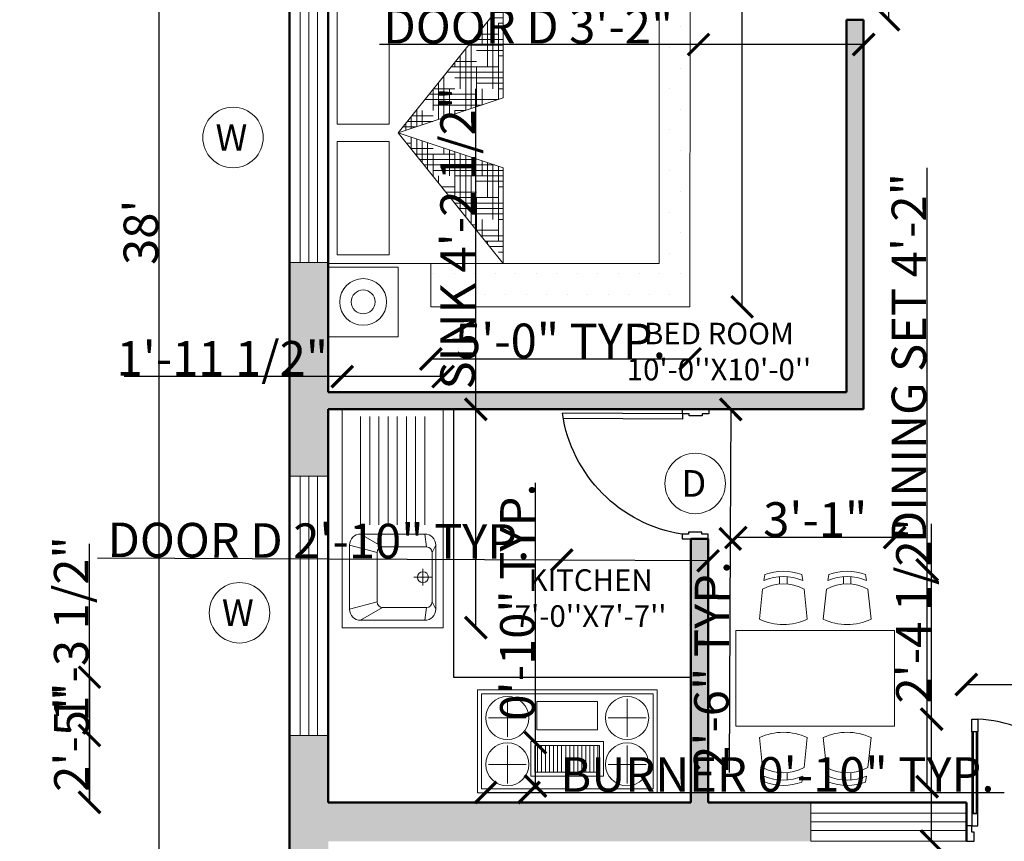
# Model space of a CAD drawing. Units: inches. Extents: x 1938 to 2373, y 1634 to 2225.
# Tile 2 of 5: x 1938 to 2166, y 1755 to 1945. Entities that reach past the tile are written whole.
import ezdxf

# ---------------------------------------------------------------- set-up
doc = ezdxf.new("R2010")
doc.units = ezdxf.units.IN
for name, color, linetype, lineweight in [('A-ANNO-DIMS', 2, 'Continuous', 18), ('A-ANNO-SYMB', 7, 'Continuous', 18), ('A-AREA-IDEN', 7, 'Continuous', 18), ('A-EQPM', 8, 'Continuous', 18), ('A-EQPM-PATT', 8, 'Continuous', 13), ('A-FLOR-FIXT', 9, 'Continuous', 18), ('A-FURN', 8, 'Continuous', 18), ('A-FURN-PATT', 7, 'Continuous', 13), ('A-WALL-PATT', 82, 'Continuous', 13), ('DOOR', 30, 'Continuous', 25), ('KITCHEN', 40, 'Continuous', 25), ('MAIN DOOR', 150, 'Continuous', 25), ('WALL', 7, 'Continuous', 50), ('WINDOW', 150, 'Continuous', 18)]:
    doc.layers.add(name, color=color, linetype=linetype, lineweight=lineweight)
doc.layers.add('A-Glaz', color=92, linetype='Continuous')
doc.styles.get("Standard").update_dxf_attribs({"font": 'arial.ttf'})
doc.dimstyles.get("Standard").update_dxf_attribs({"dimtxt": 8, "dimasz": 5, "dimexe": 0.18, "dimexo": 0.0625, "dimgap": 0.09, "dimtad": 1, "dimdec": 1, "dimzin": 0, "dimdsep": 46, "dimlunit": 4, "dimtxsty": 'Standard', "dimblk": 'ARCHTICK', "dimcen": 0.09, "dimse1": 1, "dimse2": 1, "dimadec": 0, "dimazin": 0, "dimtfac": 1, "dimtdec": 1, "dimtofl": 0, "dimtmove": 0, "dimatfit": 3, "dimfxl": 1, "dimtolj": 1, "dimtzin": 0, "dimarcsym": 0})

# ---------------------------------------------------------------- blocks, each defined once
blk = doc.blocks.new('A$C13CE0A17')
at = {"layer": 'A-Glaz'}
for p, q in [((0.01, 0.61), (0.01, 0.08)), ((0.03, 0.08), (0.03, 0.61))]:
    blk.add_line(p, q, dxfattribs=at)
blk.add_lwpolyline([(1.4, 0.08), (1.4, 0.61), (1.42, 0.61), (1.42, 0.08)], close=True, dxfattribs=at)
at = {"layer": 'MAIN DOOR'}
for p, q in [((0, 0.61), (0, 0.69)), ((0, 0.69), (0.04, 0.69)), ((0.04, 0.69), (0.04, 0.61)), ((0, 0.61), (0, 0.08)), ((0.04, 0.61), (0, 0.61)), ((0.04, 0.61), (0, 0.61)), ((0.03, 0.61), (0.01, 0.61)), ((0.04, 0.08), (0.04, 0.61)), ((0, 0.08), (0, 0)), ((0.04, 0.08), (0, 0.08)), ((0, 0.08), (0.04, 0.08)), ((0.01, 0.08), (0.03, 0.08)), ((0.04, 0), (0.04, 0.08)), ((-0.035, 0), (-0.035, -0.1)), ((0, 0), (-0.035, 0)), ((0, 0), (0.04, 0)), ((0, -0.04), (0, 0)), ((0.015, -0.04), (0, -0.04)), ((0.015, -0.05), (0.015, -0.04)), ((0.015, -0.1), (0.015, -0.05)), ((-0.035, -0.1), (0.015, -0.1))]:
    blk.add_line(p, q, dxfattribs=at)
for points in [[(1.39, 0.69), (1.39, 0.61), (1.43, 0.61), (1.43, 0.69)], [(1.39, 0.08), (1.39, 0.61), (1.43, 0.61), (1.43, 0.08)], [(1.39, 0), (1.39, 0.08), (1.43, 0.08), (1.43, 0)], [(1.43, 0), (1.465, 0), (1.465, -0.1), (1.415, -0.1), (1.415, -0.05), (1.415, -0.04), (1.43, -0.04)]]:
    blk.add_lwpolyline(points, close=True, dxfattribs=at)
blk.add_arc((1.3872, 0.017), 0.673, 89.76573, 181.44381, dxfattribs=at)
blk.add_ellipse((0.0389, 0.0511), major_axis=(0.6669, -0.1217), ratio=0.940794, start_param=0.11153, end_param=1.73917, dxfattribs=at)
blk = doc.blocks.new('table-23')
at = {"color": 0, "linetype": 'ByBlock'}
for p, q in [((-0.9, -1.4923), (-0.9, 0)), ((-0.9, 0), (0, 0)), ((0, -1.4923), (0, 0)), ((-1.3677, -0.2639), (-1.4237, -0.2726)), ((-1.0062, -0.2211), (-1.2862, -0.2511)), ((0.1062, -0.2211), (0.3862, -0.2511)), ((0.4677, -0.2639), (0.5237, -0.2726)), ((-1.4049, -0.4111), (-1.3347, -0.4111)), ((0.5049, -0.4111), (0.4347, -0.4111)), ((-1.4049, -0.4811), (-1.3347, -0.4811)), ((0.5049, -0.4811), (0.4347, -0.4811)), ((-1.3677, -0.6284), (-1.4237, -0.6197)), ((-1.0062, -0.6711), (-1.2862, -0.6411)), ((0.1062, -0.6711), (0.3862, -0.6411)), ((0.4677, -0.6284), (0.5237, -0.6197)), ((-1.0062, -0.8211), (-1.2862, -0.8511)), ((0.1062, -0.8211), (0.3862, -0.8511)), ((-1.3677, -0.8639), (-1.4237, -0.8726)), ((0.4677, -0.8639), (0.5237, -0.8726)), ((-1.4049, -1.0111), (-1.3347, -1.0111)), ((0.5049, -1.0111), (0.4347, -1.0111)), ((-1.4049, -1.0811), (-1.3347, -1.0811)), ((0.5049, -1.0811), (0.4347, -1.0811)), ((-1.3677, -1.2284), (-1.4237, -1.2197)), ((-1.0062, -1.2711), (-1.2862, -1.2411)), ((0.1062, -1.2711), (0.3862, -1.2411)), ((0.4677, -1.2284), (0.5237, -1.2197)), ((-0.9, -1.4923), (0, -1.4923))]:
    blk.add_line(p, q, dxfattribs=at)
for centre, radius, start, end in [((-0.9765, -0.4461), 0.4797, 158.78869, 201.21131), ((-0.9558, -0.4461), 0.4505, 156.13443, 203.86557), ((-0.931, -0.4461), 0.4053, 151.23721, 208.76279), ((-1.4875, -0.4461), 0.5312, 334.94238, 25.05762), ((0.5875, -0.4461), 0.5312, 154.94238, 205.05762), ((0.031, -0.4461), 0.4053, 331.23721, 28.76279), ((0.0558, -0.4461), 0.4505, 336.13443, 23.86557), ((0.0765, -0.4461), 0.4797, 338.78869, 21.21131), ((-1.4875, -1.0461), 0.5312, 334.94238, 25.05762), ((0.5875, -1.0461), 0.5312, 154.94238, 205.05762), ((-0.9765, -1.0461), 0.4797, 158.78869, 201.21131), ((-0.9558, -1.0461), 0.4505, 156.13443, 203.86557), ((-0.931, -1.0461), 0.4053, 151.23721, 208.76279), ((0.031, -1.0461), 0.4053, 331.23721, 28.76279), ((0.0558, -1.0461), 0.4505, 336.13443, 23.86557), ((0.0765, -1.0461), 0.4797, 338.78869, 21.21131)]:
    blk.add_arc(centre, radius, start, end, dxfattribs=at)
blk = doc.blocks.new('AP0B07')
for p, q in [((33.6, 96), (33.6, 978.8)), ((72, 96), (72, 972.3)), ((0, 96), (0, -96)), ((33.6, 96), (0, 96)), ((33.6, 48), (33.6, 96)), ((48, 48), (33.6, 48)), ((48, -48), (48, 48)), ((33.6, -96), (33.6, -48)), ((33.6, -48), (48, -48)), ((0, -96), (33.6, -96))]:
    blk.add_line(p, q)
blk.add_lwpolyline([(33.6, 96), (72, 96)])
blk.add_lwpolyline([(950, 96), (950, -96), (916.4, -96), (916.4, -48), (902, -48), (902, 48), (916.4, 48), (916.4, 96)], close=True)
blk.add_arc((-123.6, -61.2), 1051.8, 8.59637, 81.40363)
blk = doc.blocks.new('*X5')
at = {"color": 0}
for p, q in [((20.25, 14.8125), (20.2772, 14.8125)), ((20.1875, 14.75), (20.1875, 14.7669)), ((20.199, 14.7812), (20.2772, 14.7812)), ((20.1487, 14.7188), (20.2772, 14.7188)), ((20.1562, 14.625), (20.1562, 14.7281)), ((20.1739, 14.75), (20.2772, 14.75)), ((20.25, 14.3194), (20.25, 14.75)), ((20.0938, 14.375), (20.0938, 14.6504)), ((20.0984, 14.6562), (20.125, 14.6562)), ((20.1236, 14.6875), (20.25, 14.6875)), ((20.125, 14.5), (20.125, 14.6893)), ((20.0625, 14.2573), (20.0625, 14.6116)), ((20.125, 14.5938), (20.2772, 14.5938)), ((20.2188, 14.3091), (20.2188, 14.625)), ((20.25, 14.625), (20.2772, 14.625)), ((19.9979, 14.5312), (20.2772, 14.5312)), ((20.023, 14.5625), (20.2772, 14.5625)), ((20.0312, 14.2469), (20.0312, 14.5727)), ((19.9727, 14.5), (20.25, 14.5)), ((20, 14.2366), (20, 14.5)), ((20.1875, 14.2987), (20.1875, 14.5)), ((19.9062, 14.375), (19.9062, 14.4174)), ((19.9225, 14.4375), (20, 14.4375)), ((19.9476, 14.4688), (20.125, 14.4688)), ((20.25, 14.4375), (20.2772, 14.4375)), ((19.875, 14.25), (19.875, 14.3785)), ((19.9688, 14.2262), (19.9688, 14.375)), ((20, 14.375), (20.2772, 14.375)), ((20.125, 14.4062), (20.2772, 14.4062)), ((20.1562, 14.2884), (20.1562, 14.375)), ((19.8125, 14.1744), (19.8125, 14.3008)), ((19.8219, 14.3125), (20.2291, 14.3125)), ((19.8438, 14.1848), (19.8438, 14.3397)), ((19.875, 14.3438), (20.2772, 14.3438)), ((19.7716, 14.25), (20, 14.25)), ((19.7812, 14.1641), (19.7812, 14.262)), ((19.7967, 14.2812), (20.125, 14.2812)), ((19.9375, 14.2159), (19.9375, 14.25)), ((19.7213, 14.1875), (19.75, 14.1875)), ((19.7465, 14.2188), (19.875, 14.2188)), ((19.75, 14.1537), (19.75, 14.2231)), ((19.7018, 14.0938), (19.7786, 14.0938)), ((19.7188, 14.0726), (19.7188, 14.1136)), ((19.75, 14.0338), (19.75, 14.1032)), ((19.7812, 13.9949), (19.7812, 14.0929)), ((19.8125, 14), (19.8125, 14.0825)), ((19.7269, 14.0625), (19.8728, 14.0625)), ((19.752, 14.0312), (19.875, 14.0312)), ((19.9062, 13.8396), (19.9062, 14.0514)), ((19.9375, 13.8007), (19.9375, 14.0411)), ((19.9688, 13.875), (19.9688, 14.0307)), ((20, 14), (20, 14.0204)), ((19.875, 13.8784), (19.875, 14)), ((19.875, 13.9688), (20.1557, 13.9688)), ((20, 14), (20.0614, 14)), ((20.0625, 13.6454), (20.0625, 13.9996)), ((20.0938, 13.625), (20.0938, 13.9893)), ((20.125, 13.75), (20.125, 13.9789)), ((20.1562, 13.875), (20.1562, 13.9686)), ((19.8275, 13.9375), (20.25, 13.9375)), ((19.8526, 13.9062), (20.125, 13.9062)), ((20.25, 13.5), (20.25, 13.9375)), ((19.8777, 13.875), (20, 13.875)), ((20.0312, 13.6842), (20.0312, 13.875)), ((20.2188, 13.4511), (20.2188, 13.875)), ((20.25, 13.875), (20.2772, 13.875)), ((20, 13.8125), (20.2772, 13.8125)), ((20.125, 13.8438), (20.2772, 13.8438)), ((19.9532, 13.7812), (20.2772, 13.7812)), ((19.9783, 13.75), (20.25, 13.75)), ((20, 13.723), (20, 13.75)), ((20.1875, 13.49), (20.1875, 13.75)), ((20.0035, 13.7188), (20.125, 13.7188)), ((20.25, 13.6875), (20.2772, 13.6875)), ((20.0789, 13.625), (20.2772, 13.625)), ((20.125, 13.6562), (20.2772, 13.6562)), ((20.1562, 13.5288), (20.1562, 13.625)), ((20.104, 13.5938), (20.2772, 13.5938)), ((20.1292, 13.5625), (20.25, 13.5625)), ((20.2046, 13.4688), (20.2772, 13.4688)), ((20.25, 13.5), (20.2772, 13.5)), ((20.2297, 13.4375), (20.2772, 13.4375)), ((20.2549, 13.4062), (20.2772, 13.4062))]:
    blk.add_line(p, q, dxfattribs=at)
blk = doc.blocks.new('MAT-P13')
for p, q in [((-1.17, 0), (-1.17, -0.4)), ((-1.17, 0), (-0.77, 0)), ((-0.77, 0), (-0.77, -0.4)), ((-0.75, 0), (0.75, 0)), ((-0.75, 0), (-0.75, -1.9)), ((0.75, 0), (0.75, -1.9)), ((0.77, 0), (1.17, 0)), ((0.77, 0), (0.77, -0.4)), ((1.17, 0), (1.17, -0.4)), ((-0.7, -0.05), (-0.7, -0.35)), ((-0.7, -0.05), (-0.05, -0.05)), ((-0.05, -0.35), (-0.05, -0.05)), ((0.05, -0.05), (0.7, -0.05)), ((0.05, -0.35), (0.05, -0.05)), ((0.7, -0.05), (0.7, -0.35)), ((-0.7, -0.35), (-0.05, -0.35)), ((0.05, -0.35), (0.7, -0.35)), ((-1.17, -0.4), (-0.77, -0.4)), ((-0.75, -1.0034), (0, -0.4)), ((0, -0.4), (-0.75, -1.0034)), ((0, -0.4), (-0.2, -1.0034)), ((0, -0.4), (0.2, -1.0034)), ((0, -0.4), (0.75, -1.0034)), ((0.77, -0.4), (1.17, -0.4)), ((-0.75, -1.0034), (-0.2, -1.0034)), ((0.2, -1.0034), (0.75, -1.0034)), ((0.75, -1.9), (-0.75, -1.9))]:
    blk.add_line(p, q)
for points in [[(0.8468, -0.0814), (1.0932, -0.0814), (1.0932, -0.3186), (0.8468, -0.3186)], [(0.9015, -0.1361), (1.0385, -0.1361), (1.0385, -0.2639), (0.9015, -0.2639)]]:
    blk.add_lwpolyline(points, close=True)
for radius in [0.1342, 0.0686]:
    blk.add_circle((-0.97, -0.2), radius)
at = {"xscale": -1, "rotation": 90}
blk.add_blockref('*X5', (14.1285, 19.2738), dxfattribs=at)
blk = doc.blocks.new('KK')
for p, q in [((0, 0.55), (0, 0)), ((1.19, 0.55), (0, 0.55)), ((1.19, 0), (1.19, 0.55)), ((0.1, 0.51), (0.14, 0.36)), ((0.45, 0.51), (0.1, 0.51)), ((0.41, 0.36), (0.45, 0.51)), ((0.11, 0.33), (0.04, 0.45)), ((0.04, 0.45), (0.04, 0.1)), ((0.44, 0.33), (0.51, 0.45)), ((0.51, 0.1), (0.51, 0.45)), ((0.56, 0.45), (1.15, 0.45)), ((0.56, 0.4), (1.15, 0.4)), ((0.11, 0.09), (0.11, 0.33)), ((0.14, 0.36), (0.41, 0.36)), ((0.44, 0.33), (0.44, 0.09)), ((0.56, 0.35), (1.15, 0.35)), ((0.56, 0.3), (1.15, 0.3)), ((0.56, 0.25), (1.15, 0.25)), ((0.56, 0.2), (1.15, 0.2)), ((0.23, 0.11), (0.32, 0.11)), ((0.275, 0.06), (0.275, 0.16)), ((0.56, 0.15), (1.15, 0.15)), ((0.04, 0.1), (0.11, 0.09)), ((0.14, 0.06), (0.1, 0.04)), ((0.41, 0.06), (0.14, 0.06)), ((0.41, 0.06), (0.45, 0.04)), ((0.44, 0.09), (0.51, 0.1)), ((0.56, 0.1), (1.15, 0.1)), ((0, 0), (1.19, 0)), ((0.1, 0.04), (0.45, 0.04))]:
    blk.add_line(p, q)
blk.add_circle((0.275, 0.11), 0.03)
for centre, radius, start, end in [((0.1, 0.45), 0.06, 90, 180), ((0.45, 0.45), 0.06, 0, 90), ((0.14, 0.33), 0.03, 90, 180), ((0.41, 0.33), 0.03, 0, 90), ((0.1, 0.1), 0.06, 180, 270), ((0.14, 0.09), 0.03, 180, 270), ((0.41, 0.09), 0.03, 270, 0), ((0.45, 0.1), 0.06, 270, 0)]:
    blk.add_arc(centre, radius, start, end)
blk = doc.blocks.new('_ArchTick')
at = {"color": 0, "linetype": 'ByBlock', "const_width": 0.15}
blk.add_lwpolyline([(-0.5, -0.5), (0.5, 0.5)], dxfattribs=at)
blk = doc.blocks.new('*D13')
at = {"layer": 'A-ANNO-DIMS', "color": 0, "lineweight": -2, "transparency": 16777216}
blk.add_line((1969.98, 2123.59), (1969.98, 1667.59), dxfattribs=at)
at = {"layer": 'Defpoints', "color": 0, "transparency": 16777216}
for p in [(2000.23, 2123.59), (1969.98, 1667.59), (2000.23, 1667.59)]:
    blk.add_point(p, dxfattribs=at)
at = {"layer": 'A-ANNO-DIMS', "color": 0, "lineweight": -2, "transparency": 16777216, "xscale": 5, "yscale": 5, "zscale": 5}
for p, rotation in [((1969.98, 2123.59), 90), ((1969.98, 1667.59), 270)]:
    blk.add_blockref('_ArchTick', p, dxfattribs=dict(at, rotation=rotation))
at = {"layer": 'A-ANNO-DIMS', "color": 0, "transparency": 16777216, "insert": (1965.8, 1895.59), "char_height": 8, "attachment_point": 5, "rotation": 90}
blk.add_mtext("\\A1;38'", dxfattribs=at)
blk = doc.blocks.new('WIN-60IN')
for p, q in [((2.5, 0), (2.5, 60)), ((4.5, 0), (4.5, 60)), ((6.5, 0), (6.5, 60))]:
    blk.add_line(p, q)
blk.add_lwpolyline([(0, 0), (9, 0), (9, 60), (0, 60)], close=True)
blk = doc.blocks.new('WIN-36IN-SIDELIGHT')
for p, q in [((36, 6.5), (0, 6.5)), ((36, 4.5), (0, 4.5)), ((36, 2.5), (0, 2.5))]:
    blk.add_line(p, q)
blk.add_lwpolyline([(36, 0), (36, 9), (0, 9), (0, 0)], close=True)
blk = doc.blocks.new('TAG-WINDOW-W')
blk.add_circle((7, 7), 7)
blk.add_text('W', height=6.17).set_placement((2.93, 3.92))
blk = doc.blocks.new('TAG-DOOR-D')
blk.add_circle((7, 7), 7)
blk.add_text('D', height=6.17).set_placement((3.79, 3.92))
blk = doc.blocks.new('BURNER-10IN')
for p, q in [((5, 9.39), (5, 0.61)), ((9.39, 5), (0.61, 5))]:
    blk.add_line(p, q)
blk.add_circle((5, 5), 5)
blk = doc.blocks.new('RUG-BEDSIDE')
for p, q in [((0, 70.53), (0, 80.42)), ((0, 80.42), (60.05, 80.42)), ((60, 0), (60.05, 80.42)), ((0, 10), (0, 0)), ((0, 0), (60, 0))]:
    blk.add_line(p, q)
blk = doc.blocks.new('*D25')
at = {"layer": 'A-ANNO-DIMS', "color": 0, "lineweight": -2, "transparency": 16777216}
for p, q in [((2094.98, 1939.05), (2021.12, 1939.05)), ((2133.23, 1939.05), (2094.98, 1939.05))]:
    blk.add_line(p, q, dxfattribs=at)
at = {"layer": 'Defpoints', "color": 0, "transparency": 16777216}
for p in [(2094.98, 1944.79), (2133.23, 1944.79), (2094.98, 1939.05)]:
    blk.add_point(p, dxfattribs=at)
at = {"layer": 'A-ANNO-DIMS', "color": 0, "lineweight": -2, "transparency": 16777216, "xscale": 5, "yscale": 5, "zscale": 5}
for p, rotation in [((2094.98, 1939.05), 179.9999999999997), ((2133.23, 1939.05), 359.9999999999997)]:
    blk.add_blockref('_ArchTick', p, dxfattribs=dict(at, rotation=rotation))
at = {"layer": 'A-ANNO-DIMS', "color": 0, "transparency": 16777216, "insert": (2055.55, 1943.28), "char_height": 8, "attachment_point": 5}
blk.add_mtext('\\A1;DOOR D 3\'-2"', dxfattribs=at)
blk = doc.blocks.new('*D26')
at = {"layer": 'A-ANNO-DIMS', "color": 0, "lineweight": -2, "transparency": 16777216}
blk.add_line((2138.97, 1978.59), (2138.97, 1944.79), dxfattribs=at)
at = {"layer": 'Defpoints', "color": 0, "transparency": 16777216}
for p in [(2133.23, 1978.59), (2133.23, 1944.79), (2138.97, 1944.79)]:
    blk.add_point(p, dxfattribs=at)
at = {"layer": 'A-ANNO-DIMS', "color": 0, "lineweight": -2, "transparency": 16777216, "xscale": 5, "yscale": 5, "zscale": 5}
for p, rotation in [((2138.97, 1978.59), 90), ((2138.97, 1944.79), 270)]:
    blk.add_blockref('_ArchTick', p, dxfattribs=dict(at, rotation=rotation))
at = {"layer": 'A-ANNO-DIMS', "color": 0, "transparency": 16777216, "insert": (2134.79, 1961.69), "char_height": 8, "attachment_point": 5, "rotation": 90}
blk.add_mtext('\\A1;2\'-10"', dxfattribs=at)
blk = doc.blocks.new('*D27')
at = {"layer": 'A-ANNO-DIMS', "color": 0, "lineweight": -2, "transparency": 16777216}
for p, q in [((2063.29, 1819.68), (1955.73, 1820.16)), ((2097.21, 1819.52), (2063.29, 1819.68))]:
    blk.add_line(p, q, dxfattribs=at)
at = {"layer": 'Defpoints', "color": 0, "transparency": 16777216}
for p in [(2063.32, 1824.76), (2097.23, 1824.61), (2063.29, 1819.68)]:
    blk.add_point(p, dxfattribs=at)
at = {"layer": 'A-ANNO-DIMS', "color": 0, "lineweight": -2, "transparency": 16777216, "xscale": 5, "yscale": 5, "zscale": 5}
for p, rotation in [((2063.29, 1819.68), 179.7433741265147), ((2097.21, 1819.52), 359.7433741265147)]:
    blk.add_blockref('_ArchTick', p, dxfattribs=dict(at, rotation=rotation))
at = {"layer": 'A-ANNO-DIMS', "color": 0, "transparency": 16777216, "insert": (2007.03, 1824.16), "char_height": 8, "attachment_point": 5, "rotation": 359.7434}
blk.add_mtext('\\A1;DOOR D 2\'-10" TYP.', dxfattribs=at)
blk = doc.blocks.new('*D28')
at = {"layer": 'A-ANNO-DIMS', "color": 0, "lineweight": -2, "transparency": 16777216}
for p, q in [((2102.45, 1854.56), (2102.32, 1824.59)), ((2102.32, 1824.59), (2102.07, 1770.51))]:
    blk.add_line(p, q, dxfattribs=at)
at = {"layer": 'Defpoints', "color": 0, "transparency": 16777216}
for p in [(2097.36, 1854.59), (2097.23, 1824.61), (2102.32, 1824.59)]:
    blk.add_point(p, dxfattribs=at)
at = {"layer": 'A-ANNO-DIMS', "color": 0, "lineweight": -2, "transparency": 16777216, "xscale": 5, "yscale": 5, "zscale": 5}
for p, rotation in [((2102.45, 1854.56), 89.74337412651481), ((2102.32, 1824.59), 269.7433741265148)]:
    blk.add_blockref('_ArchTick', p, dxfattribs=dict(at, rotation=rotation))
at = {"layer": 'A-ANNO-DIMS', "color": 0, "transparency": 16777216, "insert": (2098.01, 1795.07), "char_height": 8, "attachment_point": 5, "rotation": 89.7434}
blk.add_mtext('\\A1;2\'-6" TYP.', dxfattribs=at)
blk = doc.blocks.new('*D31')
at = {"layer": 'A-ANNO-DIMS', "color": 0, "lineweight": -2, "transparency": 16777216}
for p, q in [((2045.7, 1765.89), (2055.7, 1765.89)), ((2055.7, 1765.89), (2165.8, 1765.89))]:
    blk.add_line(p, q, dxfattribs=at)
at = {"layer": 'Defpoints', "color": 0, "transparency": 16777216}
for p in [(2045.7, 1767.39), (2055.7, 1767.39), (2055.7, 1765.89)]:
    blk.add_point(p, dxfattribs=at)
at = {"layer": 'A-ANNO-DIMS', "color": 0, "lineweight": -2, "transparency": 16777216, "xscale": 5, "yscale": 5, "zscale": 5, "rotation": 180}
blk.add_blockref('_ArchTick', (2045.7, 1765.89), dxfattribs=at)
at = {"layer": 'A-ANNO-DIMS', "color": 0, "lineweight": -2, "transparency": 16777216, "xscale": 5, "yscale": 5, "zscale": 5}
blk.add_blockref('_ArchTick', (2055.7, 1765.89), dxfattribs=at)
at = {"layer": 'A-ANNO-DIMS', "color": 0, "transparency": 16777216, "insert": (2113.25, 1770.06), "char_height": 8, "attachment_point": 5}
blk.add_mtext('\\A1;BURNER 0\'-10" TYP.', dxfattribs=at)
blk = doc.blocks.new('*D32')
at = {"layer": 'A-ANNO-DIMS', "color": 0, "lineweight": -2, "transparency": 16777216}
for p, q in [((2057.2, 1777.39), (2057.2, 1837.55)), ((2057.2, 1767.39), (2057.2, 1777.39))]:
    blk.add_line(p, q, dxfattribs=at)
at = {"layer": 'Defpoints', "color": 0, "transparency": 16777216}
for p in [(2055.7, 1777.39), (2057.2, 1777.39), (2055.7, 1767.39)]:
    blk.add_point(p, dxfattribs=at)
at = {"layer": 'A-ANNO-DIMS', "color": 0, "lineweight": -2, "transparency": 16777216, "xscale": 5, "yscale": 5, "zscale": 5}
for p, rotation in [((2057.2, 1777.39), 90), ((2057.2, 1767.39), 270)]:
    blk.add_blockref('_ArchTick', p, dxfattribs=dict(at, rotation=rotation))
at = {"layer": 'A-ANNO-DIMS', "color": 0, "transparency": 16777216, "insert": (2053.02, 1809.97), "char_height": 8, "attachment_point": 5, "rotation": 90}
blk.add_mtext('\\A1;0\'-10" TYP.', dxfattribs=at)
blk = doc.blocks.new('*D43')
at = {"layer": 'A-ANNO-DIMS', "color": 0, "lineweight": -2, "transparency": 16777216}
for p, q in [((2105.09, 1958.74), (2105.09, 2111.08)), ((2105.09, 1878.32), (2105.09, 1958.74))]:
    blk.add_line(p, q, dxfattribs=at)
at = {"layer": 'Defpoints', "color": 0, "transparency": 16777216}
for p in [(2093.02, 1958.74), (2105.09, 1958.74), (2093.02, 1878.32)]:
    blk.add_point(p, dxfattribs=at)
at = {"layer": 'A-ANNO-DIMS', "color": 0, "lineweight": -2, "transparency": 16777216, "xscale": 5, "yscale": 5, "zscale": 5}
for p, rotation in [((2105.09, 1958.74), 90), ((2105.09, 1878.32), 270)]:
    blk.add_blockref('_ArchTick', p, dxfattribs=dict(at, rotation=rotation))
at = {"layer": 'A-ANNO-DIMS', "color": 0, "transparency": 16777216, "insert": (2100.86, 2037.41), "char_height": 8, "attachment_point": 5, "rotation": 90}
blk.add_mtext('\\A1;BEDSIDE RUG 6\'-8 1/2" TYP.', dxfattribs=at)
blk = doc.blocks.new('*D44')
at = {"layer": 'A-ANNO-DIMS', "color": 0, "lineweight": -2, "transparency": 16777216}
blk.add_line((2032.97, 1866.26), (2093.02, 1866.26), dxfattribs=at)
at = {"layer": 'Defpoints', "color": 0, "transparency": 16777216}
for p in [(2032.97, 1878.32), (2093.02, 1878.32), (2093.02, 1866.26)]:
    blk.add_point(p, dxfattribs=at)
at = {"layer": 'A-ANNO-DIMS', "color": 0, "lineweight": -2, "transparency": 16777216, "xscale": 5, "yscale": 5, "zscale": 5, "rotation": 180}
blk.add_blockref('_ArchTick', (2032.97, 1866.26), dxfattribs=at)
at = {"layer": 'A-ANNO-DIMS', "color": 0, "lineweight": -2, "transparency": 16777216, "xscale": 5, "yscale": 5, "zscale": 5}
blk.add_blockref('_ArchTick', (2093.02, 1866.26), dxfattribs=at)
at = {"layer": 'A-ANNO-DIMS', "color": 0, "transparency": 16777216, "insert": (2063, 1870.43), "char_height": 8, "attachment_point": 5}
blk.add_mtext('\\A1;5\'-0" TYP.', dxfattribs=at)
blk = doc.blocks.new('*D45')
at = {"layer": 'A-ANNO-DIMS', "color": 0, "lineweight": -2, "transparency": 16777216}
for p, q in [((2157.02, 1790.89), (2210.64, 1790.89)), ((2210.64, 1790.89), (2332.92, 1790.89))]:
    blk.add_line(p, q, dxfattribs=at)
at = {"layer": 'Defpoints', "color": 0, "transparency": 16777216}
for p in [(2210.64, 1790.89), (2157.02, 1782.85), (2210.64, 1782.85)]:
    blk.add_point(p, dxfattribs=at)
at = {"layer": 'A-ANNO-DIMS', "color": 0, "lineweight": -2, "transparency": 16777216, "xscale": 5, "yscale": 5, "zscale": 5, "rotation": 180}
blk.add_blockref('_ArchTick', (2157.02, 1790.89), dxfattribs=at)
at = {"layer": 'A-ANNO-DIMS', "color": 0, "lineweight": -2, "transparency": 16777216, "xscale": 5, "yscale": 5, "zscale": 5}
blk.add_blockref('_ArchTick', (2210.64, 1790.89), dxfattribs=at)
at = {"layer": 'A-ANNO-DIMS', "color": 0, "transparency": 16777216, "insert": (2274.28, 1795.12), "char_height": 8, "attachment_point": 5}
blk.add_mtext('\\A1;ENTRY DOOR 4\'-5 1/2"', dxfattribs=at)
blk = doc.blocks.new('*D46')
at = {"layer": 'A-ANNO-DIMS', "color": 0, "lineweight": -2, "transparency": 16777216}
for p, q in [((2148.98, 1782.85), (2148.98, 1828.07)), ((2148.98, 1754.59), (2148.98, 1782.85))]:
    blk.add_line(p, q, dxfattribs=at)
at = {"layer": 'Defpoints', "color": 0, "transparency": 16777216}
for p in [(2148.98, 1782.85), (2157.02, 1782.85), (2157.02, 1754.59)]:
    blk.add_point(p, dxfattribs=at)
at = {"layer": 'A-ANNO-DIMS', "color": 0, "lineweight": -2, "transparency": 16777216, "xscale": 5, "yscale": 5, "zscale": 5}
for p, rotation in [((2148.98, 1782.85), 90), ((2148.98, 1754.59), 270)]:
    blk.add_blockref('_ArchTick', p, dxfattribs=dict(at, rotation=rotation))
at = {"layer": 'A-ANNO-DIMS', "color": 0, "transparency": 16777216, "insert": (2144.75, 1807.96), "char_height": 8, "attachment_point": 5, "rotation": 90}
blk.add_mtext('\\A1;2\'-4 1/2"', dxfattribs=at)
blk = doc.blocks.new('*D47')
at = {"layer": 'A-ANNO-DIMS', "color": 0, "lineweight": -2, "transparency": 16777216}
for p, q in [((2147.93, 1817.38), (2147.93, 1910.49)), ((2147.93, 1767.23), (2147.93, 1817.38))]:
    blk.add_line(p, q, dxfattribs=at)
at = {"layer": 'Defpoints', "color": 0, "transparency": 16777216}
for p in [(2140.41, 1817.38), (2147.93, 1817.38), (2140.41, 1767.23)]:
    blk.add_point(p, dxfattribs=at)
at = {"layer": 'A-ANNO-DIMS', "color": 0, "lineweight": -2, "transparency": 16777216, "xscale": 5, "yscale": 5, "zscale": 5}
for p, rotation in [((2147.93, 1817.38), 90), ((2147.93, 1767.23), 270)]:
    blk.add_blockref('_ArchTick', p, dxfattribs=dict(at, rotation=rotation))
at = {"layer": 'A-ANNO-DIMS', "color": 0, "transparency": 16777216, "insert": (2143.71, 1866.44), "char_height": 8, "attachment_point": 5, "rotation": 90}
blk.add_mtext('\\A1;DINING SET 4\'-2"', dxfattribs=at)
blk = doc.blocks.new('*D48')
at = {"layer": 'A-ANNO-DIMS', "color": 0, "lineweight": -2, "transparency": 16777216}
blk.add_line((2140.41, 1824.91), (2103.62, 1824.91), dxfattribs=at)
at = {"layer": 'Defpoints', "color": 0, "transparency": 16777216}
for p in [(2103.62, 1824.91), (2103.62, 1817.38), (2140.41, 1817.38)]:
    blk.add_point(p, dxfattribs=at)
at = {"layer": 'A-ANNO-DIMS', "color": 0, "lineweight": -2, "transparency": 16777216, "xscale": 5, "yscale": 5, "zscale": 5, "rotation": 180}
blk.add_blockref('_ArchTick', (2103.62, 1824.91), dxfattribs=at)
at = {"layer": 'A-ANNO-DIMS', "color": 0, "lineweight": -2, "transparency": 16777216, "xscale": 5, "yscale": 5, "zscale": 5}
blk.add_blockref('_ArchTick', (2140.41, 1824.91), dxfattribs=at)
at = {"layer": 'A-ANNO-DIMS', "color": 0, "transparency": 16777216, "insert": (2122.02, 1829.08), "char_height": 8, "attachment_point": 5}
blk.add_mtext('\\A1;3\'-1"', dxfattribs=at)
blk = doc.blocks.new('*D51')
at = {"layer": 'A-ANNO-DIMS', "color": 0, "lineweight": -2, "transparency": 16777216}
for p, q in [((2043.4, 1854.59), (2043.4, 1928.82)), ((2043.4, 1804.04), (2043.4, 1854.59))]:
    blk.add_line(p, q, dxfattribs=at)
at = {"layer": 'Defpoints', "color": 0, "transparency": 16777216}
for p in [(2035.81, 1854.59), (2043.4, 1854.59), (2035.81, 1804.04)]:
    blk.add_point(p, dxfattribs=at)
at = {"layer": 'A-ANNO-DIMS', "color": 0, "lineweight": -2, "transparency": 16777216, "xscale": 5, "yscale": 5, "zscale": 5}
for p, rotation in [((2043.4, 1854.59), 90), ((2043.4, 1804.04), 270)]:
    blk.add_blockref('_ArchTick', p, dxfattribs=dict(at, rotation=rotation))
at = {"layer": 'A-ANNO-DIMS', "color": 0, "transparency": 16777216, "insert": (2039.17, 1894.2), "char_height": 8, "attachment_point": 5, "rotation": 90}
blk.add_mtext('\\A1;SINK 4\'-2 1/2"', dxfattribs=at)
blk = doc.blocks.new('*D52')
at = {"layer": 'A-ANNO-DIMS', "color": 0, "lineweight": -2, "transparency": 16777216}
for p, q in [((2012.45, 1862.17), (1961.9, 1862.17)), ((2035.81, 1862.17), (2012.45, 1862.17))]:
    blk.add_line(p, q, dxfattribs=at)
at = {"layer": 'Defpoints', "color": 0, "transparency": 16777216}
for p in [(2012.45, 1862.17), (2012.45, 1854.59), (2035.81, 1854.59)]:
    blk.add_point(p, dxfattribs=at)
at = {"layer": 'A-ANNO-DIMS', "color": 0, "lineweight": -2, "transparency": 16777216, "xscale": 5, "yscale": 5, "zscale": 5, "rotation": 180}
blk.add_blockref('_ArchTick', (2012.45, 1862.17), dxfattribs=at)
at = {"layer": 'A-ANNO-DIMS', "color": 0, "lineweight": -2, "transparency": 16777216, "xscale": 5, "yscale": 5, "zscale": 5}
blk.add_blockref('_ArchTick', (2035.81, 1862.17), dxfattribs=at)
at = {"layer": 'A-ANNO-DIMS', "color": 0, "transparency": 16777216, "insert": (1984.68, 1866.39), "char_height": 8, "attachment_point": 5}
blk.add_mtext('\\A1;1\'-11 1/2"', dxfattribs=at)
blk = doc.blocks.new('*D62')
at = {"layer": 'A-ANNO-DIMS', "color": 0, "lineweight": -2, "transparency": 16777216}
for p, q in [((1953.9, 1779.09), (1953.9, 1823.42)), ((1953.9, 1763.59), (1953.9, 1779.09))]:
    blk.add_line(p, q, dxfattribs=at)
at = {"layer": 'Defpoints', "color": 0, "transparency": 16777216}
for p in [(1953.9, 1779.09), (2009.23, 1779.09), (2009.23, 1763.59)]:
    blk.add_point(p, dxfattribs=at)
at = {"layer": 'A-ANNO-DIMS', "color": 0, "lineweight": -2, "transparency": 16777216, "xscale": 5, "yscale": 5, "zscale": 5}
for p, rotation in [((1953.9, 1779.09), 90), ((1953.9, 1763.59), 270)]:
    blk.add_blockref('_ArchTick', p, dxfattribs=dict(at, rotation=rotation))
at = {"layer": 'A-ANNO-DIMS', "color": 0, "transparency": 16777216, "insert": (1949.67, 1803.75), "char_height": 8, "attachment_point": 5, "rotation": 90}
blk.add_mtext('\\A1;1\'-3 1/2"', dxfattribs=at)
blk = doc.blocks.new('*D67')
at = {"layer": 'A-ANNO-DIMS', "color": 0, "lineweight": -2, "transparency": 16777216}
blk.add_line((2038.23, 1641.54), (2009.23, 1641.54), dxfattribs=at)
at = {"layer": 'Defpoints', "color": 0, "transparency": 16777216}
for p in [(2038.23, 1792.59), (2009.23, 1763.59), (2009.23, 1641.54)]:
    blk.add_point(p, dxfattribs=at)
at = {"layer": 'A-ANNO-DIMS', "color": 0, "lineweight": -2, "transparency": 16777216, "xscale": 5, "yscale": 5, "zscale": 5, "rotation": 180}
blk.add_blockref('_ArchTick', (2009.23, 1641.54), dxfattribs=at)
at = {"layer": 'A-ANNO-DIMS', "color": 0, "lineweight": -2, "transparency": 16777216, "xscale": 5, "yscale": 5, "zscale": 5}
blk.add_blockref('_ArchTick', (2038.23, 1641.54), dxfattribs=at)
at = {"layer": 'A-ANNO-DIMS', "color": 0, "transparency": 16777216, "insert": (2023.73, 1645.71), "char_height": 8, "attachment_point": 5}
blk.add_mtext('\\A1;2\'-5"', dxfattribs=at)
blk = doc.blocks.new('*D68')
at = {"layer": 'A-ANNO-DIMS', "color": 0, "lineweight": -2, "transparency": 16777216}
blk.add_line((1953.9, 1792.59), (1953.9, 1763.59), dxfattribs=at)
at = {"layer": 'Defpoints', "color": 0, "transparency": 16777216}
for p in [(2038.23, 1792.59), (1953.9, 1763.59), (2009.23, 1763.59)]:
    blk.add_point(p, dxfattribs=at)
at = {"layer": 'A-ANNO-DIMS', "color": 0, "lineweight": -2, "transparency": 16777216, "xscale": 5, "yscale": 5, "zscale": 5}
for p, rotation in [((1953.9, 1792.59), 90), ((1953.9, 1763.59), 270)]:
    blk.add_blockref('_ArchTick', p, dxfattribs=dict(at, rotation=rotation))
at = {"layer": 'A-ANNO-DIMS', "color": 0, "transparency": 16777216, "insert": (1949.72, 1778.09), "char_height": 8, "attachment_point": 5, "rotation": 90}
blk.add_mtext('\\A1;2\'-5"', dxfattribs=at)
blk = doc.blocks.new('*D69')
at = {"layer": 'A-ANNO-DIMS', "color": 0, "lineweight": -2, "transparency": 16777216}
blk.add_line((2043.75, 1641.54), (2085.39, 1641.54), dxfattribs=at)
at = {"layer": 'Defpoints', "color": 0, "transparency": 16777216}
for p in [(2043.75, 1765.79), (2085.39, 1765.79), (2085.39, 1641.54)]:
    blk.add_point(p, dxfattribs=at)
at = {"layer": 'A-ANNO-DIMS', "color": 0, "lineweight": -2, "transparency": 16777216, "xscale": 5, "yscale": 5, "zscale": 5, "rotation": 180}
blk.add_blockref('_ArchTick', (2043.75, 1641.54), dxfattribs=at)
at = {"layer": 'A-ANNO-DIMS', "color": 0, "lineweight": -2, "transparency": 16777216, "xscale": 5, "yscale": 5, "zscale": 5}
blk.add_blockref('_ArchTick', (2085.39, 1641.54), dxfattribs=at)
at = {"layer": 'A-ANNO-DIMS', "color": 0, "transparency": 16777216, "insert": (2064.57, 1645.76), "char_height": 8, "attachment_point": 5}
blk.add_mtext('\\A1;3\'-5 1/2"', dxfattribs=at)
blk = doc.blocks.new('*D70')
at = {"layer": 'A-ANNO-DIMS', "color": 0, "lineweight": -2, "transparency": 16777216}
blk.add_line((2318.07, 1765.79), (2318.07, 1789.65), dxfattribs=at)
at = {"layer": 'Defpoints', "color": 0, "transparency": 16777216}
for p in [(2085.39, 1789.65), (2318.07, 1789.65), (2085.39, 1765.79)]:
    blk.add_point(p, dxfattribs=at)
at = {"layer": 'A-ANNO-DIMS', "color": 0, "lineweight": -2, "transparency": 16777216, "xscale": 5, "yscale": 5, "zscale": 5}
for p, rotation in [((2318.07, 1789.65), 90), ((2318.07, 1765.79), 270)]:
    blk.add_blockref('_ArchTick', p, dxfattribs=dict(at, rotation=rotation))
at = {"layer": 'A-ANNO-DIMS', "color": 0, "transparency": 16777216, "insert": (2313.89, 1777.72), "char_height": 8, "attachment_point": 5, "rotation": 90}
blk.add_mtext('\\A1;2\'-0"', dxfattribs=at)

msp = doc.modelspace()

# ---------------------------------------------------------------- hatches: boundary and pattern name
at = {"layer": 'A-EQPM-PATT'}
h = msp.add_hatch(dxfattribs=at)
h.set_pattern_fill('ANSI31', color=256, scale=0.2947164, angle=45, style=0)
h.paths.add_polyline_path([(2057.08, 1770.57), (2072.05, 1770.57), (2072.05, 1776.74), (2057.08, 1776.74)])
at = {"layer": 'A-FURN-PATT', "transparency": 33554585}
h = msp.add_hatch(dxfattribs=at)
h.set_pattern_fill('DOTS', color=256, scale=3)
h.paths.add_polyline_path([(2093.02, 2088.74), (2032.97, 2088.74), (2032.97, 2078.85), (2085.9, 2078.85), (2085.9, 2018.32), (2032.97, 2018.32), (2032.97, 2008.32), (2092.97, 2008.32)])
h.paths.add_polyline_path([(2093.02, 1958.74), (2032.97, 1958.74), (2032.97, 1948.85), (2085.9, 1948.85), (2085.9, 1888.32), (2032.97, 1888.32), (2032.97, 1878.32), (2092.97, 1878.32)])
at = {"layer": 'A-WALL-PATT', "transparency": 33554585}
h = msp.add_hatch(color=256, dxfattribs=at)
h.dxf.hatch_style = 1
h.paths.add_polyline_path([(2076.23, 2123.59), (2000.23, 2123.59), (2000.23, 2078.59), (2009.23, 2078.59), (2009.23, 2078.85), (2009.23, 2114.59), (2076.23, 2114.59)])
h.paths.add_polyline_path([(2219.23, 2123.59), (2136.23, 2123.59), (2136.23, 2114.59), (2203.23, 2114.59), (2203.23, 2085.96), (2207.23, 2085.96), (2207.23, 2114.59), (2219.23, 2114.59)])
h.paths.add_polyline_path([(2276.23, 2123.59), (2255.23, 2123.59), (2255.23, 2114.59), (2262.62, 2114.59), (2267.23, 2114.59), (2267.23, 2050.59), (2203.23, 2050.59), (2203.23, 1978.59), (2207.23, 1978.59), (2207.23, 1984.65), (2207.23, 2046.59), (2267.23, 2046.59), (2267.23, 2032.59), (2276.23, 2032.59)])
h.paths.add_polyline_path([(2009.23, 2018.59), (2000.23, 2018.59), (2000.23, 1948.59), (2009.23, 1948.59), (2009.23, 1948.85), (2009.23, 1978.59), (2126.4, 1978.59), (2126.4, 1978.59), (2133.23, 1978.59), (2166.7, 1978.59), (2166.7, 1982.59), (2009.23, 1982.59)])
h.paths.add_polyline_path([(2276.23, 1996.59), (2267.23, 1996.59), (2267.23, 1982.59), (2237.23, 1982.59), (2237.23, 1978.59), (2267.23, 1978.59), (2267.23, 1901.32), (2276.23, 1901.32)])
h.paths.add_polyline_path([(2133.23, 1944.79), (2129.23, 1944.79), (2129.23, 1858.59), (2009.23, 1858.59), (2009.23, 1888.59), (2000.23, 1888.59), (2000.23, 1839.09), (2009.23, 1839.09), (2009.23, 1854.59), (2091.31, 1854.59), (2091.31, 1854.61), (2097.36, 1854.59), (2133.23, 1854.59)])
h.paths.add_polyline_path([(2121.02, 1763.59), (2097.23, 1763.59), (2097.23, 1824.61), (2093.23, 1824.61), (2093.23, 1763.59), (2009.23, 1763.59), (2009.23, 1779.09), (2000.23, 1779.09), (2000.23, 1739.59), (2009.23, 1739.59), (2009.23, 1754.59), (2121.02, 1754.59)])
h.paths.add_polyline_path([(2108.23, 1676.59), (2009.23, 1676.59), (2009.23, 1691.59), (2000.23, 1691.59), (2000.23, 1667.59), (2108.23, 1667.59)])
h.paths.add_polyline_path([(2276.23, 1841.32), (2267.23, 1841.32), (2267.23, 1763.59), (2246.64, 1763.59), (2246.64, 1754.59), (2276.23, 1754.59)])

# ---------------------------------------------------------------- linework, layer by layer
at = {"layer": 'A-EQPM'}
for p, q in [((2043.75, 1765.79), (2043.75, 1789.65)), ((2043.75, 1789.65), (2085.39, 1789.65)), ((2044.68, 1766.73), (2044.68, 1788.72)), ((2044.68, 1788.72), (2084.45, 1788.72)), ((2084.45, 1788.72), (2084.45, 1766.73)), ((2085.39, 1789.65), (2085.39, 1765.79)), ((2057.55, 1780.38), (2057.55, 1786.93)), ((2057.55, 1786.93), (2064.57, 1786.93)), ((2071.59, 1786.93), (2064.57, 1786.93)), ((2071.59, 1780.38), (2071.59, 1786.93)), ((2057.55, 1780.38), (2064.57, 1780.38)), ((2071.59, 1780.38), (2064.57, 1780.38)), ((2056.15, 1777.68), (2064.57, 1777.68)), ((2056.15, 1769.63), (2056.15, 1777.68)), ((2057.08, 1776.74), (2064.57, 1776.74)), ((2057.08, 1770.57), (2057.08, 1776.74)), ((2072.99, 1777.68), (2064.57, 1777.68)), ((2072.05, 1776.74), (2064.57, 1776.74)), ((2072.05, 1770.57), (2072.05, 1776.74)), ((2072.99, 1769.63), (2072.99, 1777.68)), ((2057.08, 1770.57), (2064.57, 1770.57)), ((2072.05, 1770.57), (2064.57, 1770.57)), ((2056.15, 1769.63), (2064.57, 1769.63)), ((2072.99, 1769.63), (2064.57, 1769.63)), ((2085.39, 1765.79), (2043.75, 1765.79)), ((2084.45, 1766.73), (2044.68, 1766.73))]:
    msp.add_line(p, q, dxfattribs=at)
at = {"layer": 'KITCHEN'}
for p, q in [((2038.23, 1854.59), (2038.23, 1792.59)), ((2038.23, 1792.59), (2093.23, 1792.59))]:
    msp.add_line(p, q, dxfattribs=at)
at = {"layer": 'WALL'}
for p, q in [((2000.23, 2123.59), (2000.23, 1667.59)), ((2009.23, 1978.59), (2009.23, 1858.59)), ((2129.23, 1944.79), (2129.23, 1858.59)), ((2129.23, 1944.79), (2133.23, 1944.79)), ((2133.23, 1944.79), (2133.23, 1854.59)), ((2009.23, 1858.59), (2129.23, 1858.59)), ((2009.23, 1854.59), (2133.23, 1854.59)), ((2009.23, 1854.59), (2009.23, 1763.59)), ((2093.23, 1824.61), (2093.23, 1763.59)), ((2093.23, 1824.61), (2097.23, 1824.61)), ((2097.23, 1824.61), (2097.23, 1763.59)), ((2009.23, 1763.59), (2093.23, 1763.59)), ((2097.23, 1763.59), (2157.02, 1763.59)), ((2157.02, 1754.59), (2157.02, 1763.59))]:
    msp.add_line(p, q, dxfattribs=at)

# ---------------------------------------------------------------- block references
at = {"layer": 'A-ANNO-SYMB'}
for name, p in [('TAG-WINDOW-W', (1980.16, 1910.51)), ('TAG-DOOR-D', (2087.2, 1830.43)), ('TAG-WINDOW-W', (1981.65, 1800.49))]:
    msp.add_blockref(name, p, dxfattribs=at)
at = {"layer": 'A-EQPM'}
for p, rotation in [((2055.7, 1778.14), 90.00000000003266), ((2073.44, 1777.39), 269.999999999997)]:
    msp.add_blockref('BURNER-10IN', p, dxfattribs=dict(at, rotation=rotation))
for p in [(2073.44, 1778.14), (2045.7, 1767.39)]:
    msp.add_blockref('BURNER-10IN', p, dxfattribs=at)
at = {"layer": 'A-FLOR-FIXT', "xscale": 42.47797856393942, "yscale": 42.47797856393942, "zscale": 42.47797856393942, "rotation": 90}
msp.add_blockref('KK', (2035.81, 1804.04), dxfattribs=at)
at = {"layer": 'A-FURN', "rotation": 90}
for name, p, xscale, yscale, zscale in [('MAT-P13', (2009.23, 1918.59), 40.35297549234498, 40.35297549234498, 40.35297549234498), ('table-23', (2103.62, 1803.4), 24.65510308357859, 24.65510308357859, 24.65510308357859)]:
    msp.add_blockref(name, p, dxfattribs=dict(at, xscale=xscale, yscale=yscale, zscale=zscale))
at = {"layer": 'A-FURN'}
msp.add_blockref('RUG-BEDSIDE', (2032.97, 1878.32), dxfattribs=at)
at = {"layer": 'DOOR', "xscale": -0.0315520352976369, "yscale": 0.0315520352976369, "zscale": 0.0315520352976369, "rotation": 89.74337412651481}
msp.add_blockref('AP0B07', (2094.33, 1854.6), dxfattribs=at)
at = {"layer": 'MAIN DOOR', "xscale": 35.74477478846772, "yscale": 35.74477478846772, "zscale": 35.74477478846772}
msp.add_blockref('A$C13CE0A17', (2158.27, 1758.16), dxfattribs=at)
at = {"layer": 'WINDOW'}
for name, p in [('WIN-60IN', (2000.23, 1888.58)), ('WIN-60IN', (2000.23, 1779.09)), ('WIN-36IN-SIDELIGHT', (2121.02, 1754.59))]:
    msp.add_blockref(name, p, dxfattribs=at)

# ---------------------------------------------------------------- texts
at = {"layer": 'A-AREA-IDEN', "char_height": 5, "attachment_point": 1}
for s, insert in [("\\pxqc;BED ROOM\\P10'-0''X10'-0''", (2067.96, 1874.63)), ("\\pxqc;KITCHEN\\P7'-0''X7'-7''", (2038.23, 1817.56))]:
    msp.add_mtext_dynamic_manual_height_columns(s, width=63.5129, gutter_width=30.83, heights=[0], dxfattribs=dict(at, insert=insert))

# ---------------------------------------------------------------- dimensions: what is measured, and where the dimension line sits
at = {"layer": 'A-ANNO-DIMS'}
for base, p1, p2, angle, override, picture, middle in [((1969.98, 1667.59), (2000.23, 2123.59), (2000.23, 1667.59), 90, {"dimclrd": 0, "dimclre": 0, "dimclrt": 0}, '*D13', (1965.8, 1895.59)), ((2138.97, 1944.79), (2133.23, 1978.59), (2133.23, 1944.79), 270, {"dimdec": 1, "dimlfac": 1, "dimrnd": 0, "dimzin": 1, "dimdsep": 46, "dimlunit": 4, "dimfrac": 2}, '*D26', (2134.79, 1961.69)), ((2012.45, 1862.17), (2035.81, 1854.59), (2012.45, 1854.59), 180, {"dimdec": 1, "dimlfac": 1, "dimrnd": 0, "dimzin": 1, "dimdsep": 46, "dimlunit": 4, "dimfrac": 2}, '*D52', (1984.68, 1866.39)), ((2103.62, 1824.91), (2140.41, 1817.38), (2103.62, 1817.38), 180, {"dimdec": 1, "dimlfac": 1, "dimrnd": 0, "dimzin": 1, "dimdsep": 46, "dimlunit": 4, "dimfrac": 2}, '*D48', (2122.02, 1829.08)), ((2148.98, 1782.85), (2157.02, 1754.59), (2157.02, 1782.85), 90, {"dimdec": 1, "dimlfac": 1, "dimrnd": 0, "dimzin": 1, "dimdsep": 46, "dimlunit": 4, "dimfrac": 2}, '*D46', (2144.75, 1807.96)), ((1953.9, 1779.09), (2009.23, 1763.59), (2009.23, 1779.09), 90, {"dimdec": 1, "dimlfac": 1, "dimrnd": 0, "dimzin": 1, "dimdsep": 46, "dimlunit": 4, "dimfrac": 2}, '*D62', (1949.67, 1803.75)), ((1953.9, 1763.59), (2038.23, 1792.59), (2009.23, 1763.59), 90, {"dimdec": 1, "dimlfac": 1, "dimrnd": 0, "dimzin": 1, "dimdsep": 46, "dimlunit": 4, "dimfrac": 2}, '*D68', (1949.72, 1778.09)), ((2318.07, 1789.65), (2085.39, 1765.79), (2085.39, 1789.65), 90, {"dimdec": 1, "dimlfac": 1, "dimrnd": 0, "dimzin": 1, "dimdsep": 46, "dimlunit": 4, "dimfrac": 2}, '*D70', (2313.89, 1777.72))]:
    dim = msp.add_linear_dim(base=base, p1=p1, p2=p2, angle=angle, dimstyle='Standard', override=override, dxfattribs=at)
    dim.commit()
    dim.dimension.update_dxf_attribs({"geometry": picture, "text_midpoint": middle})
for base, p1, p2, angle, text, picture, middle in [((2105.09, 1958.74), (2093.02, 1878.32), (2093.02, 1958.74), 90, 'BEDSIDE RUG <> TYP.', '*D43', (2100.86, 2037.41)), ((2094.9804, 1939.0478), (2133.2288, 1944.785), (2094.9804, 1944.785), 180, 'DOOR D <>', '*D25', (2055.5521, 1943.2796)), ((2043.3961, 1854.5853), (2035.8138, 1804.0365), (2035.8138, 1854.5853), 90, 'SINK <>', '*D51', (2039.1697, 1894.2046)), ((2147.9344, 1817.3838), (2140.4116, 1767.2318), (2140.4116, 1817.3838), 90, 'DINING SET <>', '*D47', (2143.708, 1866.4384)), ((2102.32, 1824.59), (2097.36, 1854.59), (2097.23, 1824.61), 269.7434, '<> TYP.', '*D28', (2098.01, 1795.07)), ((2063.29, 1819.68), (2097.23, 1824.61), (2063.32, 1824.76), 179.7434, 'DOOR D <> TYP.', '*D27', (2007.03, 1824.16)), ((2057.2, 1777.39), (2055.7, 1767.39), (2055.7, 1777.39), 90, '<> TYP.', '*D32', (2053.02, 1809.97))]:
    dim = msp.add_linear_dim(base=base, p1=p1, p2=p2, angle=angle, text=text, dimstyle='Standard', override={"dimdec": 1, "dimlfac": 1, "dimrnd": 0, "dimzin": 1, "dimdsep": 46, "dimlunit": 4, "dimfrac": 2}, dxfattribs=at)
    dim.commit()
    dim.dimension.update_dxf_attribs({"geometry": picture, "text_midpoint": middle})
for base, p1, p2, text, picture, middle in [((2093.0226, 1866.2572), (2032.9725, 1878.3205), (2093.0226, 1878.3205), '<> TYP.', '*D44', (2062.9975, 1870.4318)), ((2210.64, 1790.89), (2157.02, 1782.85), (2210.64, 1782.85), 'ENTRY DOOR <>', '*D45', (2274.28, 1795.12)), ((2055.7, 1765.89), (2045.7, 1767.39), (2055.7, 1767.39), 'BURNER <> TYP.', '*D31', (2113.25, 1770.06))]:
    dim = msp.add_linear_dim(base=base, p1=p1, p2=p2, text=text, dimstyle='Standard', override={"dimdec": 1, "dimlfac": 1, "dimrnd": 0, "dimzin": 1, "dimdsep": 46, "dimlunit": 4, "dimfrac": 2}, dxfattribs=at)
    dim.commit()
    dim.dimension.update_dxf_attribs({"geometry": picture, "text_midpoint": middle})
for base, p1, p2, picture, middle in [((2009.23, 1641.54), (2038.23, 1792.59), (2009.23, 1763.59), '*D67', (2023.73, 1645.71)), ((2085.39, 1641.54), (2043.75, 1765.79), (2085.39, 1765.79), '*D69', (2064.57, 1645.76))]:
    dim = msp.add_linear_dim(base=base, p1=p1, p2=p2, dimstyle='Standard', override={"dimdec": 1, "dimlfac": 1, "dimrnd": 0, "dimzin": 1, "dimdsep": 46, "dimlunit": 4, "dimfrac": 2}, dxfattribs=at)
    dim.commit()
    dim.dimension.update_dxf_attribs({"geometry": picture, "text_midpoint": middle})

doc.saveas('drawing.dxf')
